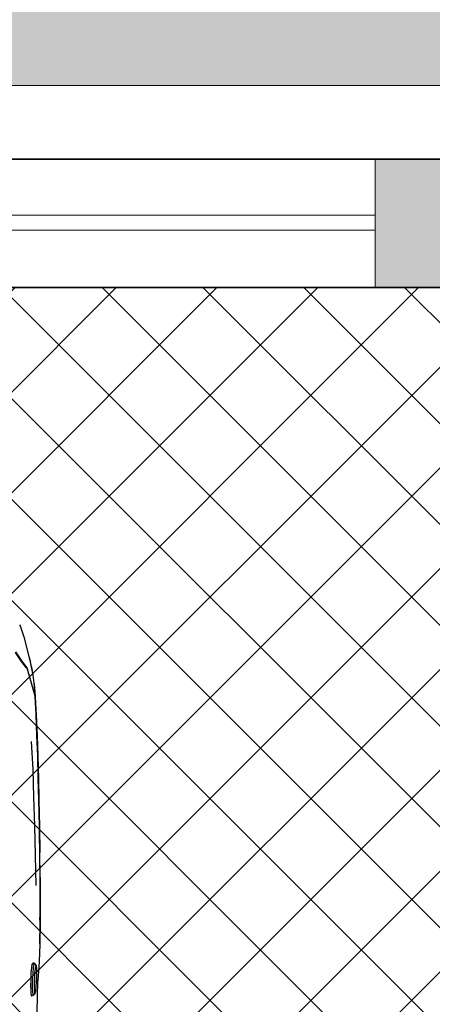
# Model space of a CAD drawing. Units: inches. Extents: x 2167 to 2589, y 1680 to 2489.
# Tile 24 of 38: x 2306 to 2335, y 1796 to 1865. Entities that reach past the tile are written whole.
import ezdxf

# ---------------------------------------------------------------- set-up
doc = ezdxf.new("R2010")
doc.units = ezdxf.units.IN
doc.header["$MEASUREMENT"] = 0
doc.layers.get('0').update_dxf_attribs({"color": 250})
for name, color, linetype, lineweight in [('A-FURN-PATT', 31, 'Continuous', 13), ('A-WALL-PATT', 250, 'Continuous', 13), ('C-PRKG-VEHS', 8, 'Continuous', 13), ('furniture', 34, 'Continuous', 18), ('L-PVMT-PATT', 252, 'Continuous', 13), ('walls', 7, 'Continuous', 35), ('windows', 141, 'Continuous', 18)]:
    doc.layers.add(name, color=color, linetype=linetype, lineweight=lineweight)
doc.layers.add('Edges', color=250, linetype='Continuous')

# ---------------------------------------------------------------- blocks, each defined once
blk = doc.blocks.new('FABRIC SOFA 4S')
at = {"layer": 'furniture'}
blk.add_line((0, -51), (0, 51), dxfattribs=at)
blk = doc.blocks.new('Nissan Qashqai pl')
at = {"layer": 'Edges'}
for p, q in [((7.7673, 12.7961), (7.8058, 12.8055)), ((7.8087, 12.8062), (7.7848, 12.8012)), ((7.8676, 12.8123), (7.7998, 12.7928)), ((7.8012, 12.7929), (7.8681, 12.8121)), ((7.8106, 12.8065), (7.8087, 12.8062)), ((7.8106, 12.8065), (7.8107, 12.8065)), ((7.8107, 12.8065), (7.8363, 12.8097)), ((7.8363, 12.8097), (7.8676, 12.8123)), ((7.8363, 12.8097), (7.8381, 12.81)), ((7.8381, 12.81), (7.87, 12.8126)), ((7.8676, 12.8123), (7.8681, 12.8121)), ((7.869, 12.8124), (7.8681, 12.8121)), ((7.9137, 12.815), (7.869, 12.8124)), ((7.87, 12.8126), (7.9151, 12.8152)), ((7.9658, 12.8172), (7.9137, 12.815)), ((7.9151, 12.8152), (7.9668, 12.8174)), ((8.016, 12.8189), (7.9658, 12.8172)), ((7.9668, 12.8174), (8.0168, 12.8191)), ((7.9803, 12.803), (8.05, 12.8066)), ((8.0713, 12.8205), (8.016, 12.8189)), ((8.0168, 12.8191), (8.0718, 12.8207)), ((8.05, 12.8066), (8.1176, 12.8087)), ((8.1249, 12.8218), (8.0713, 12.8205)), ((8.0718, 12.8207), (8.1251, 12.822)), ((8.1176, 12.8087), (8.1888, 12.8107)), ((8.1901, 12.8232), (8.1249, 12.8218)), ((8.1251, 12.822), (8.1902, 12.8233)), ((8.1888, 12.8107), (8.2622, 12.8125)), ((8.2094, 12.8235), (8.1901, 12.8232)), ((8.1902, 12.8233), (8.2543, 12.8243)), ((8.2543, 12.8243), (8.2094, 12.8235)), ((8.2543, 12.8243), (8.2094, 12.8235)), ((8.2544, 12.8242), (8.2094, 12.8235)), ((8.2693, 12.8245), (8.2543, 12.8243)), ((8.3166, 12.8249), (8.2544, 12.8242)), ((8.2622, 12.8125), (8.3356, 12.8141)), ((8.3098, 12.825), (8.2693, 12.8245)), ((8.3159, 12.825), (8.2693, 12.8245)), ((8.3159, 12.825), (8.3098, 12.825)), ((8.3159, 12.825), (8.3163, 12.825)), ((8.3163, 12.825), (8.3657, 12.8252)), ((8.3163, 12.825), (8.3597, 12.8252)), ((8.3764, 12.8251), (8.3166, 12.8249)), ((8.3597, 12.8252), (8.3657, 12.8252)), ((8.3657, 12.8252), (8.3663, 12.8252)), ((8.3663, 12.8252), (8.3747, 12.8252)), ((8.3764, 12.8251), (8.3663, 12.8252)), ((8.3747, 12.8252), (8.3757, 12.8252)), ((8.3757, 12.8252), (8.4282, 12.8249)), ((8.4069, 12.8249), (8.3764, 12.8251)), ((8.4219, 12.8246), (8.4069, 12.8249)), ((8.4292, 12.8248), (8.4069, 12.8249)), ((8.4282, 12.8249), (8.4799, 12.8239)), ((8.4799, 12.8239), (8.4292, 12.8248)), ((8.4799, 12.8239), (8.4811, 12.8239)), ((8.4811, 12.8239), (8.5241, 12.8222)), ((8.5241, 12.8222), (8.5707, 12.8193)), ((8.5287, 12.8112), (8.5269, 12.8082)), ((8.5322, 12.8047), (8.5269, 12.8082)), ((8.5287, 12.8112), (8.5331, 12.815)), ((8.5287, 12.8112), (8.531, 12.8095)), ((8.531, 12.8095), (8.5385, 12.8079)), ((8.5322, 12.8047), (8.5375, 12.8036)), ((8.5347, 12.8159), (8.5331, 12.815)), ((8.5331, 12.815), (8.5346, 12.8138)), ((8.5346, 12.8138), (8.5406, 12.8125)), ((8.5407, 12.8167), (8.5347, 12.8159)), ((8.5385, 12.8079), (8.5518, 12.8066)), ((8.5406, 12.8125), (8.5526, 12.8114)), ((8.5527, 12.8169), (8.5407, 12.8167)), ((8.5518, 12.8066), (8.568, 12.8059)), ((8.5526, 12.8114), (8.5681, 12.8107)), ((8.5682, 12.8164), (8.5527, 12.8169)), ((8.568, 12.8059), (8.5842, 12.8057)), ((8.5681, 12.8107), (8.5836, 12.8104)), ((8.5837, 12.8154), (8.5682, 12.8164)), ((8.5707, 12.8193), (8.5719, 12.8193)), ((8.6489, 12.8179), (8.5719, 12.8193)), ((8.5836, 12.8104), (8.5957, 12.8107)), ((8.5958, 12.8141), (8.5837, 12.8154)), ((8.5842, 12.8057), (8.5974, 12.8061)), ((8.5957, 12.8107), (8.6017, 12.8114)), ((8.6018, 12.8129), (8.5958, 12.8141)), ((8.5974, 12.8061), (8.6049, 12.8069)), ((8.6017, 12.8114), (8.6032, 12.8121)), ((8.6032, 12.8121), (8.6018, 12.8129)), ((8.6073, 12.808), (8.6032, 12.8121)), ((8.6049, 12.8069), (8.6073, 12.808)), ((8.6073, 12.808), (8.6093, 12.804)), ((7.6953, 12.7753), (7.7223, 12.7851)), ((7.7223, 12.7851), (7.7673, 12.7961)), ((7.7673, 12.7961), (7.7848, 12.8012)), ((7.7814, 12.7791), (7.7991, 12.7923)), ((7.7984, 12.7909), (7.7828, 12.7793)), ((7.7835, 12.8007), (7.7835, 12.8007)), ((7.7865, 12.8013), (7.7866, 12.8013)), ((7.7936, 12.8029), (7.7977, 12.8038)), ((7.7976, 12.792), (7.7991, 12.7923)), ((7.8007, 12.7926), (7.7984, 12.7909)), ((7.7991, 12.7923), (7.7998, 12.7928)), ((7.7995, 12.7924), (7.8007, 12.7926)), ((7.8012, 12.7929), (7.8007, 12.7926)), ((8.5375, 12.8036), (8.5513, 12.8023)), ((8.5513, 12.8023), (8.5678, 12.8016)), ((8.5678, 12.8016), (8.5844, 12.8014)), ((8.5844, 12.8014), (8.5921, 12.8016)), ((8.5921, 12.8016), (8.6021, 12.8022)), ((8.6021, 12.8022), (8.6065, 12.8027)), ((8.6065, 12.8027), (8.6093, 12.804)), ((7.6926, 12.7737), (7.6953, 12.7753)), ((7.7591, 12.7641), (7.7814, 12.7791)), ((7.7828, 12.7793), (7.7606, 12.7644))]:
    blk.add_line(p, q, dxfattribs=at)
blk = doc.blocks.new('car')
blk.add_blockref('Nissan Qashqai pl', (-9.7433, -11.9151))
blk = doc.blocks.new('carr')
blk.add_blockref('car', (0.5124, -0.007))

msp = doc.modelspace()

# ---------------------------------------------------------------- hatches: boundary and pattern name
at = {"layer": 'A-FURN-PATT'}
h = msp.add_hatch(color=256, dxfattribs=at)
h.dxf.hatch_style = 1
h.paths.add_polyline_path([(2263.924, 1886.408), (2263.924, 1869.74), (2282.825, 1869.74), (2282.825, 1886.408)])
h.paths.add_polyline_path([(2282.825, 1886.408), (2282.825, 1869.74), (2301.725, 1869.74), (2301.725, 1886.408)])
h.paths.add_polyline_path([(2301.725, 1886.408), (2301.725, 1869.74), (2320.625, 1869.74), (2320.625, 1886.408)])
h.paths.add_polyline_path([(2320.625, 1886.408), (2320.625, 1869.74), (2339.525, 1869.74), (2339.525, 1886.408)])
h.paths.add_polyline_path([(2263.924, 1869.74), (2261.245, 1864.978), (2342.204, 1864.978), (2339.525, 1869.74)])
h.paths.add_polyline_path([(2261.245, 1864.978), (2261.245, 1860.216), (2342.204, 1860.216), (2342.204, 1864.978)])
h.paths.add_polyline_path([(2258.864, 1887.202), (2258.864, 1862.597), (2261.245, 1862.597), (2261.245, 1864.978), (2263.627, 1869.211), (2263.627, 1887.202)])
h.paths.add_polyline_path([(2339.823, 1887.202), (2339.823, 1869.211), (2342.204, 1864.978), (2342.204, 1862.597), (2344.585, 1862.597), (2344.585, 1887.202)])
at = {"layer": 'A-WALL-PATT'}
h = msp.add_hatch(color=256, dxfattribs=at)
h.dxf.hatch_style = 1
h.paths.add_polyline_path([(2274.738, 1855.042), (2224.048, 1855.042), (2224.048, 2003.119), (2215.048, 2003.119), (2215.048, 1846.042), (2274.738, 1846.042)])
h.paths.add_polyline_path([(2354.886, 1855.042), (2330.895, 1855.042), (2330.895, 1846.042), (2354.773, 1846.042), (2354.773, 1852.042, -0.01877)])
h.paths.add_polyline_path([(2422.048, 1864.695), (2426.208, 1864.695), (2426.208, 1867.924), (2426.208, 1869.195), (2422.048, 1869.195), (2422.048, 1916.243), (2417.548, 1916.243), (2417.548, 1855.042), (2394.773, 1855.042), (2394.773, 1852.042), (2394.773, 1846.042), (2417.548, 1846.042), (2417.548, 1779.195), (2427.738, 1779.195), (2427.738, 1783.941), (2427.738, 1788.195), (2422.048, 1788.195)])
at = {"layer": 'L-PVMT-PATT'}
h = msp.add_hatch(dxfattribs=at)
h.set_pattern_fill('ANSI37', color=256, scale=40)
h.paths.add_polyline_path([(2417.548, 1783.695), (2417.548, 1846.042), (2239.361, 1846.042), (2239.361, 1687.695), (2369.843, 1687.695), (2369.843, 1696.695), (2375.607, 1696.695), (2416.107, 1696.695), (2417.548, 1696.695)])

# ---------------------------------------------------------------- linework, layer by layer
at = {"layer": 'walls'}
for p, q in [((2224.048, 1855.042), (2354.886, 1855.042)), ((2215.048, 1846.042), (2417.548, 1846.042))]:
    msp.add_line(p, q, dxfattribs=at)
at = {"layer": 'windows'}
for p, q in [((2330.895, 1855.042), (2274.738, 1855.042)), ((2330.895, 1846.042), (2330.895, 1855.042)), ((2274.738, 1851.135), (2330.895, 1851.135)), ((2330.895, 1851.135), (2330.895, 1850.068)), ((2330.895, 1850.068), (2274.738, 1850.068)), ((2274.738, 1846.042), (2330.895, 1846.042))]:
    msp.add_line(p, q, dxfattribs=at)

# ---------------------------------------------------------------- block references
at = {"layer": 'C-PRKG-VEHS', "xscale": 28.42784210623918, "yscale": 28.42784210623918, "zscale": 28.42784210623918, "rotation": 270}
msp.add_blockref('carr', (2281.736, 1778.659), dxfattribs=at)
at = {"layer": 'furniture', "xscale": 0.7937147270336093, "yscale": 0.7937147270336093, "zscale": 0.7937147270336093, "rotation": 90}
msp.add_blockref('FABRIC SOFA 4S', (2301.725, 1860.216), dxfattribs=at)

doc.saveas('drawing.dxf')
